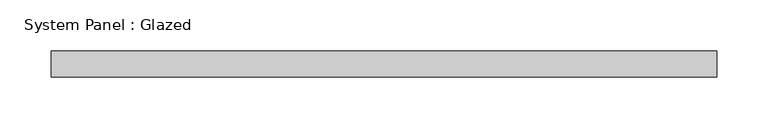
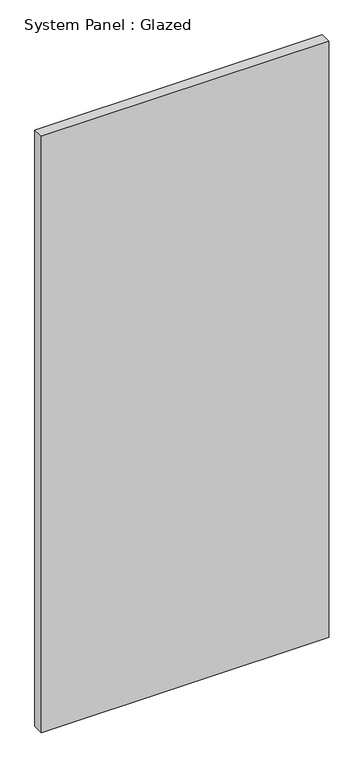
"""IFC4 building model written with IfcOpenShell, lengths in millimetres: plate geometry, System Panel : Glazed."""

from ifc_helpers import new_model, si_unit, origin, origin_with_axes, place, context, project, spatial, polyline, outline, extrude, source, transform, mapped, element, save


def system_panel_glazed_f1df731e(model_context):
    return source(origin(), model_context, "Body", "SweptSolid", [
        extrude(outline(polyline([(323.85, 19.05), (-323.85, 19.05), (-323.85, 44.45), (323.85, 44.45), (323.85, 19.05)])), origin_with_axes(), (0.0, 0.0, 1.0), 1422.4),
    ])


if __name__ == "__main__":
    model = new_model("IFC4")
    model_context = context("Model", 3, world=origin())
    ifc_project = project(units=[si_unit("LENGTHUNIT", "METRE", prefix="MILLI")], contexts=[model_context])
    site = spatial("IfcSite", under=ifc_project)
    building = spatial("IfcBuilding", under=site)
    placement = place(None, origin())
    system_panel_glazed_shape = system_panel_glazed_f1df731e(model_context)
    element("IfcPlate", 1, ObjectType="System Panel : Glazed", at=placement, inside=building, context=model_context, shape_type="MappedRepresentation", body=[
        mapped(system_panel_glazed_shape, transform((0.0, 0.0, 0.0), x_axis=(1.0, 0.0, 0.0), y_axis=(0.0, 1.0, 0.0), z_axis=(0.0, 0.0, 1.0))),
    ])
    save(model, "model.ifc")

# Revit data of these elements
# Type "System Panel : Glazed"
#   Construction Type Id = "GSP4R"
#   Analytic Construction = "1/8 in Pilkington single glazing"
#   Visual Light Transmittance = 0.9
#   Solar Heat Gain Coefficient = 0.86
#   Heat Transfer Coefficient (U) = 1.18115 BTU/(h·ft²·°F)
#   Define Thermal Properties by = 1
# Element 1 (IfcPlate, "System Panel : Glazed")
#   Materials on its faces: "Glass"
# Materials
#   "Glass": class "Glass", colour RGB 0 128 192, transparency 0.75, Description = "Soda Lime Glass", Cost = 0
